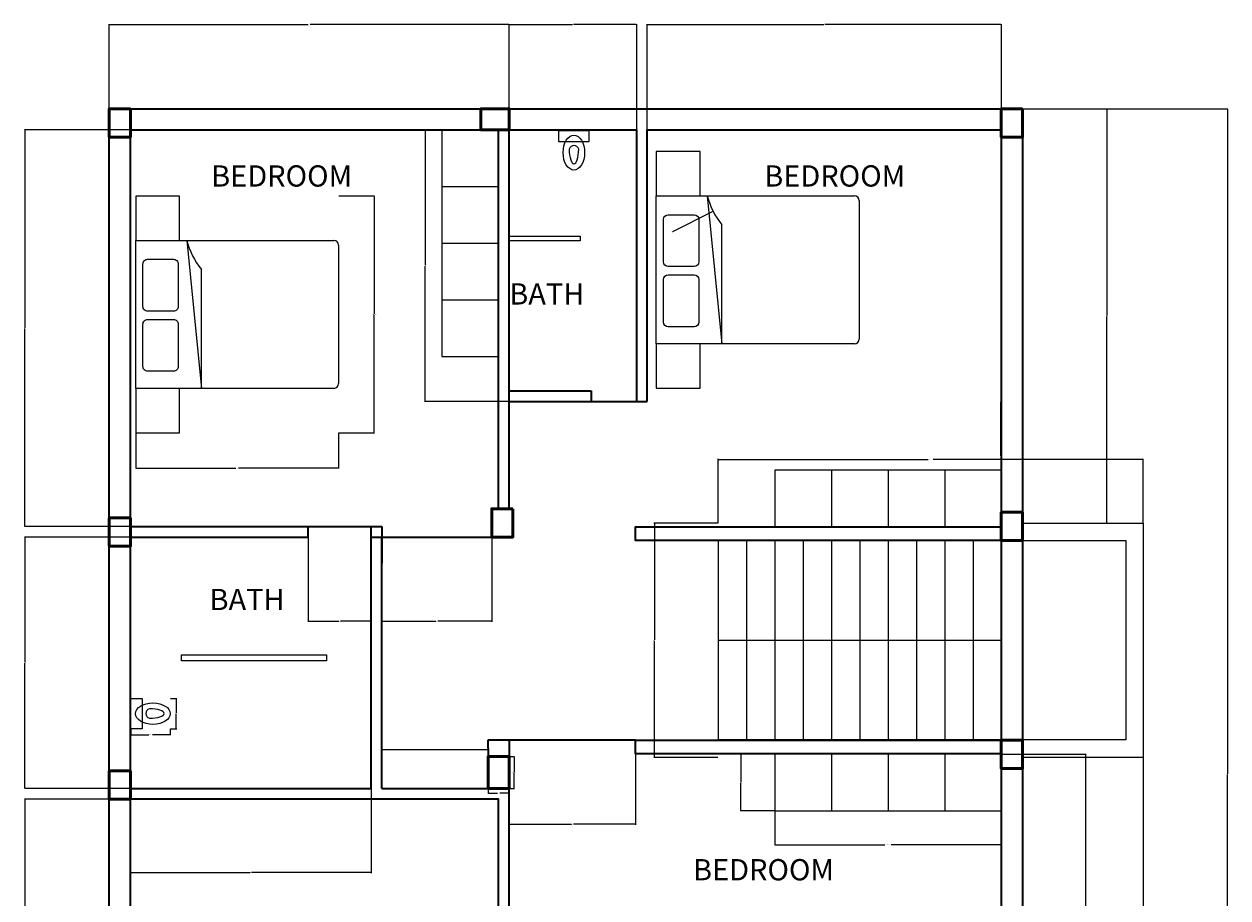
# Model space of a CAD drawing. Units: inches. Extents: x 1748 to 3019, y 1454 to 2188.
# Tile 4 of 4: x 2509 to 3019, y 1818 to 2188. Entities that reach past the tile are written whole.
import ezdxf

# ---------------------------------------------------------------- set-up
doc = ezdxf.new("R2010")
doc.units = ezdxf.units.IN
for name, color, linetype, lineweight in [('A-ANNO-DIMS', 2, 'Continuous', 18), ('A-AREA-IDEN', 134, 'Continuous', 18), ('A-COLS', 120, 'Continuous', 50), ('A-FLOR-CASE', 9, 'Continuous', 18), ('A-WALL', 7, 'Continuous', 35), ('bathroom', 54, 'Continuous', 18), ('bed', 21, 'Continuous', 18), ('cupboard', 201, 'Continuous', 18), ('stairs', 64, 'Continuous', 25)]:
    doc.layers.add(name, color=color, linetype=linetype, lineweight=lineweight)
doc.styles.get("Standard").update_dxf_attribs({"font": 'arial.ttf'})
doc.dimstyles.get("Standard").update_dxf_attribs({"dimtxt": 0.18, "dimasz": 0.18, "dimexe": 0.18, "dimexo": 0.0625, "dimgap": 0.09, "dimtad": 0, "dimtih": 1, "dimtoh": 1, "dimdec": 4, "dimzin": 0, "dimdsep": 46, "dimtxsty": 'Standard', "dimcen": 0.09, "dimadec": 0, "dimazin": 0, "dimtfac": 1, "dimtdec": 4, "dimtofl": 0, "dimtmove": 0, "dimatfit": 3, "dimfxl": 1, "dimtolj": 1, "dimtzin": 0, "dimarcsym": 0})

# ---------------------------------------------------------------- blocks, each defined once
blk = doc.blocks.new('BED-DOUBLE-NIGHTSTANDS')
for p, q in [((0, 81.51), (83.98, 81.51)), ((0, 18.79), (0, 81.51)), ((21.61, 81.51), (27.83, 18.79)), ((85.98, 79.51), (85.98, 20.79)), ((27.83, 18.79), (27.83, 69.19)), ((83.98, 18.79), (0, 18.79))]:
    blk.add_line(p, q)
for points in [[(0, 81.51), (18.52, 81.51), (18.52, 100.3), (0, 100.3)], [(0, 0), (18.52, 0), (18.52, 18.79), (0, 18.79)]]:
    blk.add_lwpolyline(points, close=True)
for points in [[(5.06, 73.49), (16.01, 73.49, -0.414214), (18.01, 71.49), (18.01, 53.51, -0.414214), (16.01, 51.51), (5.06, 51.51, -0.414214), (3.06, 53.51), (3.06, 71.49, -0.414214)], [(5.06, 47.99), (16.01, 47.99, -0.414214), (18.01, 45.99), (18.01, 28.02, -0.414214), (16.01, 26.02), (5.06, 26.02, -0.414214), (3.06, 28.02), (3.06, 45.99, -0.414214)]]:
    blk.add_lwpolyline(points, format="xyb", close=True)
for centre, radius, start, end in [((52.42, 89.31), 31.78, 194.1991, 219.2902), ((83.98, 79.51), 2, 0, 90), ((83.98, 79.51), 2, 0, 90), ((83.98, 20.79), 2, 270, 0)]:
    blk.add_arc(centre, radius, start, end)
blk = doc.blocks.new('WARDROBE-4-BAY')
for p, q in [((24, 96), (0, 96)), ((0, 96), (0, 0)), ((24, 0), (24, 96)), ((0, 72), (24, 72)), ((0, 48), (24, 48)), ((0, 24), (24, 24)), ((0, 0), (24, 0))]:
    blk.add_line(p, q)
blk = doc.blocks.new('WC-CLOSE-COUPLED')
blk.add_lwpolyline([(0, 12.82), (4.89, 12.82), (4.89, 0), (0, 0)], close=True)
blk.add_arc((8.58, 6.47), 2.15, 108.3808, 251.6192)
blk.add_ellipse((9.39, 6.41), major_axis=(7.38, 0), ratio=0.615385)
blk.add_ellipse((7.39, 6.47), major_axis=(6.81, 0), ratio=0.3, start_param=4.786849, end_param=7.779521)
blk = doc.blocks.new('STAIR-FLIGHT-LANDING')
for p, q in [((0, 91.88), (129, 91.88)), ((0, 91.88), (0, 7.38)), ((12, 91.88), (12, 7.38)), ((24, 91.88), (24, 7.38)), ((36, 91.88), (36, 7.38)), ((48, 91.88), (48, 7.38)), ((60, 91.88), (60, 7.38)), ((72, 91.88), (72, 7.38)), ((84, 91.88), (84, 7.38)), ((96, 91.88), (96, 7.38)), ((108, 91.88), (108, 7.38)), ((120, 91.88), (120, 7.38)), ((0, 49.63), (120, 49.63)), ((129, 7.38), (0, 7.38))]:
    blk.add_line(p, q)
blk.add_lwpolyline([(129, 99.26), (180.11, 99.26), (180.11, 0), (129, 0)])
blk.add_lwpolyline([(129, 91.88), (172.73, 91.88), (172.73, 7.38), (129, 7.38)], close=True)
blk = doc.blocks.new('COLUMN-9X12')
blk.add_lwpolyline([(9, 12), (9, 0), (0, 0), (0, 12)], close=True)
blk = doc.blocks.new('COLUMN-RECT-EXTENDED')
blk.add_lwpolyline([(9, 13.44), (9, 0), (0, 0), (0, 13.44)], close=True)
blk = doc.blocks.new('*D10')
at = {"layer": 'A-ANNO-DIMS', "color": 0, "lineweight": -2, "transparency": 16777216}
for p, q in [((2714.2, 1877.38), (2716.33, 1877.38)), ((2716.15, 1877.2), (2716.15, 1870.85)), ((2716.15, 1864.12), (2716.15, 1870.48)), ((2714.2, 1863.94), (2716.33, 1863.94))]:
    blk.add_line(p, q, dxfattribs=at)
at = {"layer": 'A-ANNO-DIMS', "color": 0, "transparency": 16777216}
for points in [[(2716.12, 1877.2), (2716.18, 1877.2), (2716.15, 1877.38)], [(2716.12, 1864.12), (2716.18, 1864.12), (2716.15, 1863.94)]]:
    blk.add_solid(points, dxfattribs=at)
at = {"layer": 'Defpoints', "color": 0, "transparency": 16777216}
for p in [(2714.14, 1877.38), (2716.15, 1877.38), (2714.14, 1863.94)]:
    blk.add_point(p, dxfattribs=at)
at = {"layer": 'A-ANNO-DIMS', "color": 0, "transparency": 16777216, "insert": (2716.15, 1870.66), "char_height": 0.18, "attachment_point": 5}
blk.add_mtext('\\A1;COLUMN 13 TYP.', dxfattribs=at)
blk = doc.blocks.new('*D11')
at = {"layer": 'A-ANNO-DIMS', "color": 0, "lineweight": -2, "transparency": 16777216}
for p, q in [((2705.14, 1863.88), (2705.14, 1861.74)), ((2705.32, 1861.92), (2709.18, 1861.92)), ((2713.96, 1861.92), (2710.09, 1861.92)), ((2714.14, 1863.88), (2714.14, 1861.74))]:
    blk.add_line(p, q, dxfattribs=at)
at = {"layer": 'A-ANNO-DIMS', "color": 0, "transparency": 16777216}
for points in [[(2705.32, 1861.95), (2705.32, 1861.89), (2705.14, 1861.92)], [(2713.96, 1861.95), (2713.96, 1861.89), (2714.14, 1861.92)]]:
    blk.add_solid(points, dxfattribs=at)
at = {"layer": 'Defpoints', "color": 0, "transparency": 16777216}
for p in [(2705.14, 1863.94), (2714.14, 1863.94), (2714.14, 1861.92)]:
    blk.add_point(p, dxfattribs=at)
at = {"layer": 'A-ANNO-DIMS', "color": 0, "transparency": 16777216, "insert": (2709.64, 1861.92), "char_height": 0.18, "attachment_point": 5}
blk.add_mtext('\\A1;9 TYP.', dxfattribs=at)
blk = doc.blocks.new('*D12')
at = {"layer": 'A-ANNO-DIMS', "color": 0, "lineweight": -2, "transparency": 16777216}
for p, q in [((2826.64, 1854.35), (2826.64, 1839.83)), ((2922.64, 1854.35), (2922.64, 1839.83)), ((2826.82, 1840.01), (2873.33, 1840.01)), ((2922.46, 1840.01), (2875.94, 1840.01))]:
    blk.add_line(p, q, dxfattribs=at)
at = {"layer": 'A-ANNO-DIMS', "color": 0, "transparency": 16777216}
for points in [[(2826.82, 1840.04), (2826.82, 1839.98), (2826.64, 1840.01)], [(2922.46, 1840.04), (2922.46, 1839.98), (2922.64, 1840.01)]]:
    blk.add_solid(points, dxfattribs=at)
at = {"layer": 'Defpoints', "color": 0, "transparency": 16777216}
for p in [(2826.64, 1854.41), (2922.64, 1854.41), (2922.64, 1840.01)]:
    blk.add_point(p, dxfattribs=at)
at = {"layer": 'A-ANNO-DIMS', "color": 0, "transparency": 16777216, "insert": (2874.64, 1840.01), "char_height": 0.18, "attachment_point": 5}
blk.add_mtext('\\A1;WARDROBE 96 TYP.', dxfattribs=at)
blk = doc.blocks.new('*D13')
at = {"layer": 'A-ANNO-DIMS', "color": 0, "lineweight": -2, "transparency": 16777216}
for p, q in [((2826.57, 1878.41), (2812.06, 1878.41)), ((2812.24, 1878.23), (2812.24, 1866.59)), ((2812.24, 1854.59), (2812.24, 1866.23)), ((2826.57, 1854.41), (2812.06, 1854.41))]:
    blk.add_line(p, q, dxfattribs=at)
at = {"layer": 'A-ANNO-DIMS', "color": 0, "transparency": 16777216}
for points in [[(2812.21, 1878.23), (2812.27, 1878.23), (2812.24, 1878.41)], [(2812.21, 1854.59), (2812.27, 1854.59), (2812.24, 1854.41)]]:
    blk.add_solid(points, dxfattribs=at)
at = {"layer": 'Defpoints', "color": 0, "transparency": 16777216}
for p in [(2826.64, 1878.41), (2812.24, 1854.41), (2826.64, 1854.41)]:
    blk.add_point(p, dxfattribs=at)
at = {"layer": 'A-ANNO-DIMS', "color": 0, "transparency": 16777216, "insert": (2812.24, 1866.41), "char_height": 0.18, "attachment_point": 5}
blk.add_mtext('\\A1;24 TYP.', dxfattribs=at)
blk = doc.blocks.new('*D14')
at = {"layer": 'A-ANNO-DIMS', "color": 0, "lineweight": -2, "transparency": 16777216}
for p, q in [((2553.76, 1889.14), (2553.76, 1886.51)), ((2570.53, 1889.14), (2570.53, 1886.51)), ((2553.94, 1886.69), (2561.37, 1886.69)), ((2570.35, 1886.69), (2562.92, 1886.69))]:
    blk.add_line(p, q, dxfattribs=at)
at = {"layer": 'A-ANNO-DIMS', "color": 0, "transparency": 16777216}
for points in [[(2553.94, 1886.72), (2553.94, 1886.66), (2553.76, 1886.69)], [(2570.35, 1886.72), (2570.35, 1886.66), (2570.53, 1886.69)]]:
    blk.add_solid(points, dxfattribs=at)
at = {"layer": 'Defpoints', "color": 0, "transparency": 16777216}
for p in [(2553.76, 1889.2), (2570.53, 1889.2), (2570.53, 1886.69)]:
    blk.add_point(p, dxfattribs=at)
at = {"layer": 'A-ANNO-DIMS', "color": 0, "transparency": 16777216, "insert": (2562.14, 1886.69), "char_height": 0.18, "attachment_point": 5}
blk.add_mtext('\\A1;WC 17 TYP.', dxfattribs=at)
blk = doc.blocks.new('*D15')
at = {"layer": 'A-ANNO-DIMS', "color": 0, "lineweight": -2, "transparency": 16777216}
for p, q in [((2570.59, 1902.02), (2573.22, 1902.02)), ((2573.04, 1901.84), (2573.04, 1895.8)), ((2573.04, 1889.38), (2573.04, 1895.43)), ((2570.59, 1889.2), (2573.22, 1889.2))]:
    blk.add_line(p, q, dxfattribs=at)
at = {"layer": 'A-ANNO-DIMS', "color": 0, "transparency": 16777216}
for points in [[(2573.01, 1901.84), (2573.07, 1901.84), (2573.04, 1902.02)], [(2573.01, 1889.38), (2573.07, 1889.38), (2573.04, 1889.2)]]:
    blk.add_solid(points, dxfattribs=at)
at = {"layer": 'Defpoints', "color": 0, "transparency": 16777216}
for p in [(2570.53, 1902.02), (2573.04, 1902.02), (2570.53, 1889.2)]:
    blk.add_point(p, dxfattribs=at)
at = {"layer": 'A-ANNO-DIMS', "color": 0, "transparency": 16777216, "insert": (2573.04, 1895.61), "char_height": 0.18, "attachment_point": 5}
blk.add_mtext('\\A1;13 TYP.', dxfattribs=at)
blk = doc.blocks.new('*D18')
at = {"layer": 'A-ANNO-DIMS', "color": 0, "lineweight": -2, "transparency": 16777216}
for p, q in [((2641.9, 2114.97), (2657.07, 2114.97)), ((2656.89, 2114.79), (2656.89, 2065)), ((2656.89, 2014.84), (2656.89, 2064.63)), ((2641.9, 2014.66), (2657.07, 2014.66))]:
    blk.add_line(p, q, dxfattribs=at)
at = {"layer": 'A-ANNO-DIMS', "color": 0, "transparency": 16777216}
for points in [[(2656.86, 2114.79), (2656.92, 2114.79), (2656.89, 2114.97)], [(2656.86, 2014.84), (2656.92, 2014.84), (2656.89, 2014.66)]]:
    blk.add_solid(points, dxfattribs=at)
at = {"layer": 'Defpoints', "color": 0, "transparency": 16777216}
for p in [(2641.84, 2114.97), (2656.89, 2114.97), (2641.84, 2014.66)]:
    blk.add_point(p, dxfattribs=at)
at = {"layer": 'A-ANNO-DIMS', "color": 0, "transparency": 16777216, "insert": (2656.89, 2064.81), "char_height": 0.18, "attachment_point": 5}
blk.add_mtext('\\A1;BED SET 100 TYP.', dxfattribs=at)
blk = doc.blocks.new('*D19')
at = {"layer": 'A-ANNO-DIMS', "color": 0, "lineweight": -2, "transparency": 16777216}
for p, q in [((2555.86, 2014.6), (2555.86, 1999.44)), ((2641.84, 2014.6), (2641.84, 1999.44)), ((2556.04, 1999.62), (2598.32, 1999.62)), ((2641.66, 1999.62), (2599.38, 1999.62))]:
    blk.add_line(p, q, dxfattribs=at)
at = {"layer": 'A-ANNO-DIMS', "color": 0, "transparency": 16777216}
for points in [[(2556.04, 1999.65), (2556.04, 1999.59), (2555.86, 1999.62)], [(2641.66, 1999.65), (2641.66, 1999.59), (2641.84, 1999.62)]]:
    blk.add_solid(points, dxfattribs=at)
at = {"layer": 'Defpoints', "color": 0, "transparency": 16777216}
for p in [(2555.86, 2014.66), (2641.84, 2014.66), (2641.84, 1999.62)]:
    blk.add_point(p, dxfattribs=at)
at = {"layer": 'A-ANNO-DIMS', "color": 0, "transparency": 16777216, "insert": (2598.85, 1999.62), "char_height": 0.18, "attachment_point": 5}
blk.add_mtext('\\A1;86 TYP.', dxfattribs=at)
blk = doc.blocks.new('*D20')
at = {"layer": 'A-ANNO-DIMS', "color": 0, "lineweight": -2, "transparency": 16777216}
for p, q in [((2802.64, 1976.38), (2802.64, 2003.52)), ((2802.82, 2003.34), (2891.69, 2003.34)), ((2982.56, 2003.34), (2893.69, 2003.34)), ((2982.74, 1976.38), (2982.74, 2003.52))]:
    blk.add_line(p, q, dxfattribs=at)
at = {"layer": 'A-ANNO-DIMS', "color": 0, "transparency": 16777216}
for points in [[(2802.82, 2003.37), (2802.82, 2003.31), (2802.64, 2003.34)], [(2982.56, 2003.37), (2982.56, 2003.31), (2982.74, 2003.34)]]:
    blk.add_solid(points, dxfattribs=at)
at = {"layer": 'Defpoints', "color": 0, "transparency": 16777216}
for p in [(2982.74, 2003.34), (2802.64, 1976.32), (2982.74, 1976.32)]:
    blk.add_point(p, dxfattribs=at)
at = {"layer": 'A-ANNO-DIMS', "color": 0, "transparency": 16777216, "insert": (2892.69, 2003.34), "char_height": 0.18, "attachment_point": 5}
blk.add_mtext('\\A1;STAIR 180 TYP.', dxfattribs=at)
blk = doc.blocks.new('*D21')
at = {"layer": 'A-ANNO-DIMS', "color": 0, "lineweight": -2, "transparency": 16777216}
for p, q in [((2802.57, 1976.32), (2775.44, 1976.32)), ((2775.62, 1976.14), (2775.62, 1926.87)), ((2775.62, 1877.24), (2775.62, 1926.51)), ((2802.57, 1877.06), (2775.44, 1877.06))]:
    blk.add_line(p, q, dxfattribs=at)
at = {"layer": 'A-ANNO-DIMS', "color": 0, "transparency": 16777216}
for points in [[(2775.59, 1976.14), (2775.65, 1976.14), (2775.62, 1976.32)], [(2775.59, 1877.24), (2775.65, 1877.24), (2775.62, 1877.06)]]:
    blk.add_solid(points, dxfattribs=at)
at = {"layer": 'Defpoints', "color": 0, "transparency": 16777216}
for p in [(2775.62, 1976.32), (2802.64, 1976.32), (2802.64, 1877.06)]:
    blk.add_point(p, dxfattribs=at)
at = {"layer": 'A-ANNO-DIMS', "color": 0, "transparency": 16777216, "insert": (2775.62, 1926.69), "char_height": 0.18, "attachment_point": 5}
blk.add_mtext('\\A1;99 TYP.', dxfattribs=at)
blk = doc.blocks.new('*D44')
at = {"layer": 'A-ANNO-DIMS', "color": 0, "lineweight": -2, "transparency": 16777216}
for p, q in [((2982.74, 1877), (2982.74, 1552.06)), ((2544.64, 1587.88), (2544.64, 1552.06)), ((2544.82, 1552.24), (2763.31, 1552.24)), ((2982.56, 1552.24), (2764.07, 1552.24))]:
    blk.add_line(p, q, dxfattribs=at)
at = {"layer": 'A-ANNO-DIMS', "color": 0, "transparency": 16777216}
for points in [[(2544.82, 1552.27), (2544.82, 1552.21), (2544.64, 1552.24)], [(2982.56, 1552.27), (2982.56, 1552.21), (2982.74, 1552.24)]]:
    blk.add_solid(points, dxfattribs=at)
at = {"layer": 'Defpoints', "color": 0, "transparency": 16777216}
for p in [(2982.74, 1877.06), (2544.64, 1587.94), (2982.74, 1552.24)]:
    blk.add_point(p, dxfattribs=at)
at = {"layer": 'A-ANNO-DIMS', "color": 0, "transparency": 16777216, "insert": (2763.69, 1552.24), "char_height": 0.18, "attachment_point": 5}
blk.add_mtext('\\A1;438.1', dxfattribs=at)
blk = doc.blocks.new('*D45')
at = {"layer": 'A-ANNO-DIMS', "color": 0, "lineweight": -2, "transparency": 16777216}
for p, q in [((2931.7, 2151.94), (3018.62, 2151.94)), ((3018.44, 2151.76), (3018.44, 1870.12)), ((3018.44, 1588.12), (3018.44, 1869.76)), ((2886.7, 1587.94), (3018.62, 1587.94))]:
    blk.add_line(p, q, dxfattribs=at)
at = {"layer": 'A-ANNO-DIMS', "color": 0, "transparency": 16777216}
for points in [[(3018.41, 2151.76), (3018.47, 2151.76), (3018.44, 2151.94)], [(3018.41, 1588.12), (3018.47, 1588.12), (3018.44, 1587.94)]]:
    blk.add_solid(points, dxfattribs=at)
at = {"layer": 'Defpoints', "color": 0, "transparency": 16777216}
for p in [(2931.64, 2151.94), (3018.44, 2151.94), (2886.64, 1587.94)]:
    blk.add_point(p, dxfattribs=at)
at = {"layer": 'A-ANNO-DIMS', "color": 0, "transparency": 16777216, "insert": (3018.44, 1869.94), "char_height": 0.18, "attachment_point": 5}
blk.add_mtext('\\A1;564', dxfattribs=at)
blk = doc.blocks.new('*D46')
at = {"layer": 'A-ANNO-DIMS', "color": 0, "lineweight": -2, "transparency": 16777216}
for p, q in [((2544.64, 2152), (2544.64, 2187.82)), ((2544.82, 2187.64), (2629, 2187.64)), ((2713.96, 2187.64), (2629.77, 2187.64)), ((2714.14, 2152), (2714.14, 2187.82))]:
    blk.add_line(p, q, dxfattribs=at)
at = {"layer": 'A-ANNO-DIMS', "color": 0, "transparency": 16777216}
for points in [[(2544.82, 2187.67), (2544.82, 2187.61), (2544.64, 2187.64)], [(2713.96, 2187.67), (2713.96, 2187.61), (2714.14, 2187.64)]]:
    blk.add_solid(points, dxfattribs=at)
at = {"layer": 'Defpoints', "color": 0, "transparency": 16777216}
for p in [(2714.14, 2187.64), (2544.64, 2151.94), (2714.14, 2151.94)]:
    blk.add_point(p, dxfattribs=at)
at = {"layer": 'A-ANNO-DIMS', "color": 0, "transparency": 16777216, "insert": (2629.39, 2187.64), "char_height": 0.18, "attachment_point": 5}
blk.add_mtext('\\A1;169.5', dxfattribs=at)
blk = doc.blocks.new('*D47')
at = {"layer": 'A-ANNO-DIMS', "color": 0, "lineweight": -2, "transparency": 16777216}
for p, q in [((2714.14, 2143), (2714.14, 2187.82)), ((2714.32, 2187.64), (2740.92, 2187.64)), ((2767.96, 2187.64), (2741.35, 2187.64)), ((2768.14, 2143), (2768.14, 2187.82))]:
    blk.add_line(p, q, dxfattribs=at)
at = {"layer": 'A-ANNO-DIMS', "color": 0, "transparency": 16777216}
for points in [[(2714.32, 2187.67), (2714.32, 2187.61), (2714.14, 2187.64)], [(2767.96, 2187.67), (2767.96, 2187.61), (2768.14, 2187.64)]]:
    blk.add_solid(points, dxfattribs=at)
at = {"layer": 'Defpoints', "color": 0, "transparency": 16777216}
for p in [(2768.14, 2187.64), (2714.14, 2142.94), (2768.14, 2142.94)]:
    blk.add_point(p, dxfattribs=at)
at = {"layer": 'A-ANNO-DIMS', "color": 0, "transparency": 16777216, "insert": (2741.14, 2187.64), "char_height": 0.18, "attachment_point": 5}
blk.add_mtext('\\A1;54', dxfattribs=at)
blk = doc.blocks.new('*D48')
at = {"layer": 'A-ANNO-DIMS', "color": 0, "lineweight": -2, "transparency": 16777216}
for p, q in [((2772.64, 2143.03), (2772.64, 2187.82)), ((2772.82, 2187.64), (2847.36, 2187.64)), ((2922.46, 2187.64), (2847.92, 2187.64)), ((2922.64, 2143), (2922.64, 2187.82))]:
    blk.add_line(p, q, dxfattribs=at)
at = {"layer": 'A-ANNO-DIMS', "color": 0, "transparency": 16777216}
for points in [[(2772.82, 2187.67), (2772.82, 2187.61), (2772.64, 2187.64)], [(2922.46, 2187.67), (2922.46, 2187.61), (2922.64, 2187.64)]]:
    blk.add_solid(points, dxfattribs=at)
at = {"layer": 'Defpoints', "color": 0, "transparency": 16777216}
for p in [(2922.64, 2187.64), (2772.64, 2142.97), (2922.64, 2142.94)]:
    blk.add_point(p, dxfattribs=at)
at = {"layer": 'A-ANNO-DIMS', "color": 0, "transparency": 16777216, "insert": (2847.64, 2187.64), "char_height": 0.18, "attachment_point": 5}
blk.add_mtext('\\A1;150', dxfattribs=at)
blk = doc.blocks.new('*D49')
at = {"layer": 'A-ANNO-DIMS', "color": 0, "lineweight": -2, "transparency": 16777216}
for p, q in [((2714.07, 2142.94), (2678.26, 2142.94)), ((2678.44, 2142.76), (2678.44, 2085.59)), ((2678.44, 2028.05), (2678.44, 2085.22)), ((2714.07, 2027.87), (2678.26, 2027.87))]:
    blk.add_line(p, q, dxfattribs=at)
at = {"layer": 'A-ANNO-DIMS', "color": 0, "transparency": 16777216}
for points in [[(2678.41, 2142.76), (2678.47, 2142.76), (2678.44, 2142.94)], [(2678.41, 2028.05), (2678.47, 2028.05), (2678.44, 2027.87)]]:
    blk.add_solid(points, dxfattribs=at)
at = {"layer": 'Defpoints', "color": 0, "transparency": 16777216}
for p in [(2678.44, 2142.94), (2714.14, 2142.94), (2714.14, 2027.87)]:
    blk.add_point(p, dxfattribs=at)
at = {"layer": 'A-ANNO-DIMS', "color": 0, "transparency": 16777216, "insert": (2678.44, 2085.4), "char_height": 0.18, "attachment_point": 5}
blk.add_mtext('\\A1;115.07', dxfattribs=at)
blk = doc.blocks.new('*D50')
at = {"layer": 'A-ANNO-DIMS', "color": 0, "lineweight": -2, "transparency": 16777216}
for p, q in [((2553.57, 2142.94), (2508.76, 2142.94)), ((2508.94, 2142.76), (2508.94, 2059.12)), ((2508.94, 1975.12), (2508.94, 2058.76)), ((2553.57, 1974.94), (2508.76, 1974.94))]:
    blk.add_line(p, q, dxfattribs=at)
at = {"layer": 'A-ANNO-DIMS', "color": 0, "transparency": 16777216}
for points in [[(2508.91, 2142.76), (2508.97, 2142.76), (2508.94, 2142.94)], [(2508.91, 1975.12), (2508.97, 1975.12), (2508.94, 1974.94)]]:
    blk.add_solid(points, dxfattribs=at)
at = {"layer": 'Defpoints', "color": 0, "transparency": 16777216}
for p in [(2508.94, 2142.94), (2553.64, 2142.94), (2553.64, 1974.94)]:
    blk.add_point(p, dxfattribs=at)
at = {"layer": 'A-ANNO-DIMS', "color": 0, "transparency": 16777216, "insert": (2508.94, 2058.94), "char_height": 0.18, "attachment_point": 5}
blk.add_mtext('\\A1;168', dxfattribs=at)
blk = doc.blocks.new('*D51')
at = {"layer": 'A-ANNO-DIMS', "color": 0, "lineweight": -2, "transparency": 16777216}
for p, q in [((2553.64, 1863.88), (2553.64, 1828.06)), ((2655.64, 1863.88), (2655.64, 1828.06)), ((2553.82, 1828.24), (2604.36, 1828.24)), ((2655.46, 1828.24), (2604.91, 1828.24))]:
    blk.add_line(p, q, dxfattribs=at)
at = {"layer": 'A-ANNO-DIMS', "color": 0, "transparency": 16777216}
for points in [[(2553.82, 1828.27), (2553.82, 1828.21), (2553.64, 1828.24)], [(2655.46, 1828.27), (2655.46, 1828.21), (2655.64, 1828.24)]]:
    blk.add_solid(points, dxfattribs=at)
at = {"layer": 'Defpoints', "color": 0, "transparency": 16777216}
for p in [(2553.64, 1863.94), (2655.64, 1863.94), (2553.64, 1828.24)]:
    blk.add_point(p, dxfattribs=at)
at = {"layer": 'A-ANNO-DIMS', "color": 0, "transparency": 16777216, "insert": (2604.64, 1828.24), "char_height": 0.18, "attachment_point": 5}
blk.add_mtext('\\A1;102', dxfattribs=at)
blk = doc.blocks.new('*D52')
at = {"layer": 'A-ANNO-DIMS', "color": 0, "lineweight": -2, "transparency": 16777216}
for p, q in [((2553.57, 1970.44), (2508.76, 1970.44)), ((2508.94, 1970.26), (2508.94, 1917.37)), ((2508.94, 1864.12), (2508.94, 1917.01)), ((2553.57, 1863.94), (2508.76, 1863.94))]:
    blk.add_line(p, q, dxfattribs=at)
at = {"layer": 'A-ANNO-DIMS', "color": 0, "transparency": 16777216}
for points in [[(2508.91, 1970.26), (2508.97, 1970.26), (2508.94, 1970.44)], [(2508.91, 1864.12), (2508.97, 1864.12), (2508.94, 1863.94)]]:
    blk.add_solid(points, dxfattribs=at)
at = {"layer": 'Defpoints', "color": 0, "transparency": 16777216}
for p in [(2508.94, 1970.44), (2553.64, 1970.44), (2553.64, 1863.94)]:
    blk.add_point(p, dxfattribs=at)
at = {"layer": 'A-ANNO-DIMS', "color": 0, "transparency": 16777216, "insert": (2508.94, 1917.19), "char_height": 0.18, "attachment_point": 5}
blk.add_mtext('\\A1;106.5', dxfattribs=at)
blk = doc.blocks.new('*D53')
at = {"layer": 'A-ANNO-DIMS', "color": 0, "lineweight": -2, "transparency": 16777216}
for p, q in [((2544.57, 1859.39), (2508.76, 1859.39)), ((2508.94, 1859.21), (2508.94, 1763.6)), ((2508.94, 1667.62), (2508.94, 1763.23)), ((2544.57, 1667.44), (2508.76, 1667.44))]:
    blk.add_line(p, q, dxfattribs=at)
at = {"layer": 'A-ANNO-DIMS', "color": 0, "transparency": 16777216}
for points in [[(2508.91, 1859.21), (2508.97, 1859.21), (2508.94, 1859.39)], [(2508.91, 1667.62), (2508.97, 1667.62), (2508.94, 1667.44)]]:
    blk.add_solid(points, dxfattribs=at)
at = {"layer": 'Defpoints', "color": 0, "transparency": 16777216}
for p in [(2508.94, 1859.39), (2544.64, 1859.39), (2544.64, 1667.44)]:
    blk.add_point(p, dxfattribs=at)
at = {"layer": 'A-ANNO-DIMS', "color": 0, "transparency": 16777216, "insert": (2508.94, 1763.42), "char_height": 0.18, "attachment_point": 5}
blk.add_mtext('\\A1;191.95', dxfattribs=at)
blk = doc.blocks.new('*D55')
at = {"layer": 'A-ANNO-DIMS', "color": 0, "lineweight": -2, "transparency": 16777216}
for p, q in [((2922.7, 1878.41), (2958.52, 1878.41)), ((2958.34, 1878.23), (2958.34, 1794.11)), ((2958.34, 1709.62), (2958.34, 1793.74)), ((2922.7, 1709.44), (2958.52, 1709.44))]:
    blk.add_line(p, q, dxfattribs=at)
at = {"layer": 'A-ANNO-DIMS', "color": 0, "transparency": 16777216}
for points in [[(2958.31, 1878.23), (2958.37, 1878.23), (2958.34, 1878.41)], [(2958.31, 1709.62), (2958.37, 1709.62), (2958.34, 1709.44)]]:
    blk.add_solid(points, dxfattribs=at)
at = {"layer": 'Defpoints', "color": 0, "transparency": 16777216}
for p in [(2922.64, 1878.41), (2922.64, 1709.44), (2958.34, 1709.44)]:
    blk.add_point(p, dxfattribs=at)
at = {"layer": 'A-ANNO-DIMS', "color": 0, "transparency": 16777216, "insert": (2958.34, 1793.93), "char_height": 0.18, "attachment_point": 5}
blk.add_mtext('\\A1;168.97', dxfattribs=at)
blk = doc.blocks.new('*D61')
at = {"layer": 'A-ANNO-DIMS', "color": 0, "lineweight": -2, "transparency": 16777216}
for p, q in [((2931.7, 2151.94), (2967.52, 2151.94)), ((2967.34, 2151.76), (2967.34, 2064.31)), ((2967.34, 1976.5), (2967.34, 2063.95)), ((2931.7, 1976.32), (2967.52, 1976.32))]:
    blk.add_line(p, q, dxfattribs=at)
at = {"layer": 'A-ANNO-DIMS', "color": 0, "transparency": 16777216}
for points in [[(2967.31, 2151.76), (2967.37, 2151.76), (2967.34, 2151.94)], [(2967.31, 1976.5), (2967.37, 1976.5), (2967.34, 1976.32)]]:
    blk.add_solid(points, dxfattribs=at)
at = {"layer": 'Defpoints', "color": 0, "transparency": 16777216}
for p in [(2931.64, 2151.94), (2931.64, 1976.32), (2967.34, 1976.32)]:
    blk.add_point(p, dxfattribs=at)
at = {"layer": 'A-ANNO-DIMS', "color": 0, "transparency": 16777216, "insert": (2967.34, 2064.13), "char_height": 0.18, "attachment_point": 5}
blk.add_mtext('\\A1;175.62', dxfattribs=at)
blk = doc.blocks.new('*D62')
at = {"layer": 'A-ANNO-DIMS', "color": 0, "lineweight": -2, "transparency": 16777216}
for p, q in [((2628.91, 1970.38), (2628.91, 1934.56)), ((2655.64, 1970.38), (2655.64, 1934.56)), ((2629.09, 1934.74), (2641.88, 1934.74)), ((2655.46, 1934.74), (2642.67, 1934.74))]:
    blk.add_line(p, q, dxfattribs=at)
at = {"layer": 'A-ANNO-DIMS', "color": 0, "transparency": 16777216}
for points in [[(2629.09, 1934.77), (2629.09, 1934.71), (2628.91, 1934.74)], [(2655.46, 1934.77), (2655.46, 1934.71), (2655.64, 1934.74)]]:
    blk.add_solid(points, dxfattribs=at)
at = {"layer": 'Defpoints', "color": 0, "transparency": 16777216}
for p in [(2628.91, 1970.44), (2655.64, 1970.44), (2628.91, 1934.74)]:
    blk.add_point(p, dxfattribs=at)
at = {"layer": 'A-ANNO-DIMS', "color": 0, "transparency": 16777216, "insert": (2642.27, 1934.74), "char_height": 0.18, "attachment_point": 5}
blk.add_mtext('\\A1;26.72', dxfattribs=at)
blk = doc.blocks.new('*D63')
at = {"layer": 'A-ANNO-DIMS', "color": 0, "lineweight": -2, "transparency": 16777216}
for p, q in [((2660.14, 1970.38), (2660.14, 1934.56)), ((2706.69, 1970.38), (2706.69, 1934.56)), ((2660.32, 1934.74), (2683.01, 1934.74)), ((2706.51, 1934.74), (2683.81, 1934.74))]:
    blk.add_line(p, q, dxfattribs=at)
at = {"layer": 'A-ANNO-DIMS', "color": 0, "transparency": 16777216}
for points in [[(2660.32, 1934.77), (2660.32, 1934.71), (2660.14, 1934.74)], [(2706.51, 1934.77), (2706.51, 1934.71), (2706.69, 1934.74)]]:
    blk.add_solid(points, dxfattribs=at)
at = {"layer": 'Defpoints', "color": 0, "transparency": 16777216}
for p in [(2660.14, 1970.44), (2706.69, 1970.44), (2660.14, 1934.74)]:
    blk.add_point(p, dxfattribs=at)
at = {"layer": 'A-ANNO-DIMS', "color": 0, "transparency": 16777216, "insert": (2683.41, 1934.74), "char_height": 0.18, "attachment_point": 5}
blk.add_mtext('\\A1;46.55', dxfattribs=at)
blk = doc.blocks.new('*D64')
at = {"layer": 'A-ANNO-DIMS', "color": 0, "lineweight": -2, "transparency": 16777216}
for p, q in [((2714.14, 1884.35), (2714.14, 1848.53)), ((2767.68, 1884.35), (2767.68, 1848.53)), ((2714.32, 1848.71), (2740.51, 1848.71)), ((2767.5, 1848.71), (2741.3, 1848.71))]:
    blk.add_line(p, q, dxfattribs=at)
at = {"layer": 'A-ANNO-DIMS', "color": 0, "transparency": 16777216}
for points in [[(2714.32, 1848.74), (2714.32, 1848.68), (2714.14, 1848.71)], [(2767.5, 1848.74), (2767.5, 1848.68), (2767.68, 1848.71)]]:
    blk.add_solid(points, dxfattribs=at)
at = {"layer": 'Defpoints', "color": 0, "transparency": 16777216}
for p in [(2714.14, 1884.41), (2767.68, 1884.41), (2714.14, 1848.71)]:
    blk.add_point(p, dxfattribs=at)
at = {"layer": 'A-ANNO-DIMS', "color": 0, "transparency": 16777216, "insert": (2740.91, 1848.71), "char_height": 0.18, "attachment_point": 5}
blk.add_mtext('\\A1;53.54', dxfattribs=at)
blk = doc.blocks.new('*D69')
at = {"layer": 'A-ANNO-DIMS', "color": 0, "lineweight": -2, "transparency": 16777216}
for p, q in [((2828.77, 2122.84), (2828.95, 2122.84)), ((2828.86, 2122.75), (2828.86, 2122.93)), ((2783.45, 2099.96), (2800.32, 2108.46)), ((2783.27, 2099.96), (2783.45, 2099.96))]:
    blk.add_line(p, q, dxfattribs=at)
at = {"layer": 'A-ANNO-DIMS', "color": 0, "transparency": 16777216}
blk.add_solid([(2800.31, 2108.49), (2800.33, 2108.43), (2800.48, 2108.54)], dxfattribs=at)
at = {"layer": 'Defpoints', "color": 0, "transparency": 16777216}
for p in [(2828.86, 2122.84), (2800.48, 2108.54)]:
    blk.add_point(p, dxfattribs=at)
at = {"layer": 'A-ANNO-DIMS', "color": 0, "transparency": 16777216, "insert": (2782.6, 2099.96), "char_height": 0.18, "attachment_point": 5}
blk.add_mtext('\\A1;3X R31.78', dxfattribs=at)

msp = doc.modelspace()

# ---------------------------------------------------------------- linework, layer by layer
at = {"layer": 'A-FLOR-CASE'}
msp.add_line((2705.1292, 1880.2386), (2660.1353, 1880.2386), dxfattribs=at)
at = {"layer": 'A-WALL'}
for p, q in [((2553.6353, 2142.94), (2709.6353, 2142.94)), ((2553.6353, 1974.94), (2553.6353, 2142.94)), ((2709.6353, 1982.44), (2709.6353, 2142.94)), ((2714.1353, 2142.94), (2768.1353, 2142.94)), ((2714.1353, 2052.94), (2714.1353, 2142.94)), ((2768.1353, 2027.8673), (2768.1353, 2142.94)), ((2772.6353, 2027.8673), (2772.6353, 2142.9677)), ((2772.6353, 2142.9677), (2922.6353, 2142.9677)), ((2822.1836, 2142.94), (2822.1836, 2142.9677)), ((2922.6353, 2142.94), (2922.6353, 1709.44)), ((2714.1353, 1982.44), (2714.1353, 2052.94)), ((2714.1353, 2032.3673), (2748.8656, 2032.3673)), ((2748.8656, 2032.3673), (2748.8656, 2027.8673)), ((2714.1353, 2027.8673), (2772.6353, 2027.8673)), ((2714.1353, 2026.1397), (2714.1353, 2026.1397)), ((2553.6353, 1974.94), (2660.1353, 1974.94)), ((2628.9144, 1970.44), (2628.9144, 1974.94)), ((2655.6353, 1919.44), (2655.6353, 1974.94)), ((2660.1353, 1974.94), (2660.1353, 1959.3034)), ((2553.6353, 1970.44), (2618.1353, 1970.44)), ((2553.6353, 1919.44), (2553.6353, 1970.44)), ((2618.1353, 1970.44), (2628.9144, 1970.44)), ((2655.6353, 1970.44), (2714.1353, 1970.44)), ((2660.1353, 1919.44), (2660.1353, 1970.44)), ((2553.6353, 1863.94), (2553.6353, 1919.44)), ((2655.6353, 1863.94), (2655.6353, 1919.44)), ((2660.1353, 1863.94), (2660.1353, 1919.44)), ((2767.6791, 1884.412), (2705.1203, 1884.412)), ((2705.1203, 1884.412), (2705.1353, 1877.3845)), ((2714.1353, 1884.412), (2714.1353, 1877.3845)), ((2553.6353, 1863.94), (2655.6353, 1863.94)), ((2660.1353, 1863.94), (2714.1353, 1863.94)), ((2714.1353, 1716.94), (2714.1353, 1863.94)), ((2553.6353, 1859.44), (2709.6353, 1859.44)), ((2553.6353, 1667.44), (2553.6353, 1859.44)), ((2709.6353, 1587.94), (2709.6353, 1859.44))]:
    msp.add_line(p, q, dxfattribs=at)
msp.add_lwpolyline([(2886.6353, 1587.94), (2544.6353, 1587.94), (2544.6353, 2151.94), (2931.6353, 2151.94), (2931.6353, 1709.44)], dxfattribs=at)
for points in [[(2922.6353, 2027.8069), (2922.6353, 2027.8069), (2922.6353, 2004.8656), (2922.6353, 2004.8656)], [(2922.6353, 1968.94), (2767.6791, 1968.94), (2767.6791, 1974.7972), (2922.6353, 1974.7972)], [(2922.6353, 1878.5549), (2767.6791, 1878.5549), (2767.6791, 1884.412), (2922.6353, 1884.412)]]:
    msp.add_lwpolyline(points, close=True, dxfattribs=at)
at = {"layer": 'bathroom'}
for p, q in [((2714.1353, 2097.94), (2744.189, 2097.94)), ((2744.189, 2097.94), (2744.189, 2095.9804)), ((2744.189, 2095.9804), (2714.1353, 2095.9804))]:
    msp.add_line(p, q, dxfattribs=at)
msp.add_lwpolyline([(2575.2445, 1920.5791), (2636.6636, 1920.5791), (2636.6636, 1917.9975), (2575.2445, 1917.9975)], close=True, dxfattribs=at)
at = {"layer": 'bed'}
for p, q in [((2776.4369, 2115.0478), (2860.4191, 2115.0478)), ((2776.4369, 2052.3237), (2776.4369, 2115.0478)), ((2798.0507, 2115.0478), (2804.2632, 2052.3237)), ((2862.4191, 2113.0478), (2862.4191, 2054.3237)), ((2804.2632, 2052.3237), (2804.2632, 2102.7197)), ((2860.4191, 2052.3237), (2776.4369, 2052.3237))]:
    msp.add_line(p, q, dxfattribs=at)
for points in [[(2776.4369, 2115.0478), (2794.9604, 2115.0478), (2794.9604, 2133.8374), (2776.4369, 2133.8374)], [(2776.4369, 2033.5341), (2794.9604, 2033.5341), (2794.9604, 2052.3237), (2776.4369, 2052.3237)]]:
    msp.add_lwpolyline(points, close=True, dxfattribs=at)
for points in [[(2781.4925, 2107.021), (2792.4453, 2107.021, -0.41421356), (2794.4453, 2105.021), (2794.4453, 2087.0437, -0.41421356), (2792.4453, 2085.0437), (2781.4925, 2085.0437, -0.41421356), (2779.4925, 2087.0437), (2779.4925, 2105.021, -0.41421356)], [(2781.4925, 2081.5274), (2792.4453, 2081.5274, -0.41421356), (2794.4453, 2079.5274), (2794.4453, 2061.5501, -0.41421356), (2792.4453, 2059.5501), (2781.4925, 2059.5501, -0.41421356), (2779.4925, 2061.5501), (2779.4925, 2079.5274, -0.41421356)]]:
    msp.add_lwpolyline(points, format="xyb", close=True, dxfattribs=at)
for centre, radius, start, end in [((2828.8569, 2122.8424), 31.777, 194.199088, 219.290241), ((2860.4191, 2113.0478), 2, 0, 90), ((2860.4191, 2113.0478), 2, 0, 90), ((2860.4191, 2054.3237), 2, 270, 0)]:
    msp.add_arc(centre, radius, start, end, dxfattribs=at)

# ---------------------------------------------------------------- block references
at = {"layer": 'A-COLS'}
for name, p in [('COLUMN-9X12', (2544.6349, 2139.94)), ('COLUMN-9X12', (2922.6349, 2139.94)), ('COLUMN-9X12', (2706.6867, 1970.44)), ('COLUMN-9X12', (2922.6349, 1968.94)), ('COLUMN-9X12', (2544.6349, 1966.5724)), ('COLUMN-9X12', (2922.6349, 1872.412)), ('COLUMN-RECT-EXTENDED', (2705.1349, 1863.94)), ('COLUMN-9X12', (2544.6349, 1859.3932))]:
    msp.add_blockref(name, p, dxfattribs=at)
at = {"layer": 'A-COLS', "rotation": 270.0000000000023}
msp.add_blockref('COLUMN-9X12', (2702.1353, 2151.9404), dxfattribs=at)
at = {"layer": 'bathroom', "rotation": 269.9999999999866}
msp.add_blockref('WC-CLOSE-COUPLED', (2735.0925, 2142.7418), dxfattribs=at)
at = {"layer": 'bathroom'}
msp.add_blockref('WC-CLOSE-COUPLED', (2553.7588, 1889.2046), dxfattribs=at)
at = {"layer": 'bed'}
msp.add_blockref('BED-DOUBLE-NIGHTSTANDS', (2555.8569, 2014.663), dxfattribs=at)
at = {"layer": 'cupboard'}
msp.add_blockref('WARDROBE-4-BAY', (2685.6349, 2046.94), dxfattribs=at)
for p, rotation in [((2826.6353, 1998.7976), 269.9999999999998), ((2826.6353, 1878.4125), 270.0000000000005)]:
    msp.add_blockref('WARDROBE-4-BAY', p, dxfattribs=dict(at, rotation=rotation))
at = {"layer": 'stairs'}
msp.add_blockref('STAIR-FLIGHT-LANDING', (2802.6349, 1877.058), dxfattribs=at)

# ---------------------------------------------------------------- texts
at = {"layer": 'A-AREA-IDEN', "char_height": 9, "attachment_point": 1}
for s, width, insert in [('BEDROOM', 14.161869, (2587.8299, 2127.9529)), ('BEDROOM', 14.161869, (2822.1836, 2127.9529)), ('BATH', 60.883203, (2714.1353, 2077.9708)), ('BATH', 60.883203, (2587.1405, 1948.4764)), ('BEDROOM', 14.161869, (2791.9992, 1833.9663))]:
    msp.add_mtext_dynamic_manual_height_columns(s, width=width, gutter_width=12.5, heights=[0], dxfattribs=dict(at, insert=insert))

# ---------------------------------------------------------------- dimensions: what is measured, and where the dimension line sits
at = {"layer": 'A-ANNO-DIMS'}
for base, p1, p2, override, picture, middle in [((2714.1353, 2187.64), (2544.6353, 2151.94), (2714.1353, 2151.94), {"dimdec": 1, "dimlfac": 1, "dimrnd": 0, "dimzin": 0, "dimdsep": 46, "dimlunit": 2}, '*D46', (2629.3853, 2187.64)), ((2768.1353, 2187.64), (2714.1353, 2142.94), (2768.1353, 2142.94), {"dimdec": 0, "dimlfac": 1, "dimrnd": 0, "dimzin": 0, "dimdsep": 46, "dimlunit": 2}, '*D47', (2741.1353, 2187.64)), ((2922.6353, 2187.64), (2772.6353, 2142.9677), (2922.6353, 2142.94), {"dimdec": 0, "dimlfac": 1, "dimrnd": 0, "dimzin": 0, "dimdsep": 46, "dimlunit": 2}, '*D48', (2847.6353, 2187.64)), ((2982.7428, 1552.24), (2544.6353, 1587.94), (2982.7428, 1877.0584), {"dimdec": 1, "dimlfac": 1, "dimrnd": 0, "dimzin": 0, "dimdsep": 46, "dimlunit": 2}, '*D44', (2763.689, 1552.24))]:
    dim = msp.add_linear_dim(base=base, p1=p1, p2=p2, dimstyle='Standard', override=override, dxfattribs=at)
    dim.commit()
    dim.dimension.update_dxf_attribs({"geometry": picture, "text_midpoint": middle})
for base, p1, p2, angle, override, picture, middle in [((3018.4428, 2151.94), (2886.6353, 1587.94), (2931.6353, 2151.94), 90, {"dimdec": 0, "dimlfac": 1, "dimrnd": 0, "dimzin": 0, "dimdsep": 46, "dimlunit": 2}, '*D45', (3018.4428, 1869.94)), ((2967.3353, 1976.3216), (2931.6353, 2151.94), (2931.6353, 1976.3216), 270, {"dimdec": 2, "dimlfac": 1, "dimrnd": 0, "dimzin": 0, "dimdsep": 46, "dimlunit": 2}, '*D61', (2967.3353, 2064.1308)), ((2508.9353, 2142.94), (2553.6353, 1974.94), (2553.6353, 2142.94), 90, {"dimdec": 0, "dimlfac": 1, "dimrnd": 0, "dimzin": 0, "dimdsep": 46, "dimlunit": 2}, '*D50', (2508.9353, 2058.94)), ((2678.4353, 2142.94), (2714.1353, 2027.8673), (2714.1353, 2142.94), 90, {"dimdec": 2, "dimlfac": 1, "dimrnd": 0, "dimzin": 0, "dimdsep": 46, "dimlunit": 2}, '*D49', (2678.4353, 2085.4036)), ((2508.9353, 1970.44), (2553.6353, 1863.94), (2553.6353, 1970.44), 90, {"dimdec": 1, "dimlfac": 1, "dimrnd": 0, "dimzin": 0, "dimdsep": 46, "dimlunit": 2}, '*D52', (2508.9353, 1917.19)), ((2628.9144, 1934.74), (2655.6353, 1970.44), (2628.9144, 1970.44), 180, {"dimdec": 2, "dimlfac": 1, "dimrnd": 0, "dimzin": 0, "dimdsep": 46, "dimlunit": 2}, '*D62', (2642.2749, 1934.74)), ((2660.1353, 1934.74), (2706.6871, 1970.44), (2660.1353, 1970.44), 180, {"dimdec": 2, "dimlfac": 1, "dimrnd": 0, "dimzin": 0, "dimdsep": 46, "dimlunit": 2}, '*D63', (2683.4112, 1934.74)), ((2714.1353, 1848.712), (2767.6791, 1884.412), (2714.1353, 1884.412), 180, {"dimdec": 2, "dimlfac": 1, "dimrnd": 0, "dimzin": 0, "dimdsep": 46, "dimlunit": 2}, '*D64', (2740.9072, 1848.712)), ((2958.3353, 1709.44), (2922.6353, 1878.412), (2922.6353, 1709.44), 270, {"dimdec": 2, "dimlfac": 1, "dimrnd": 0, "dimzin": 0, "dimdsep": 46, "dimlunit": 2}, '*D55', (2958.3353, 1793.926)), ((2553.6353, 1828.24), (2655.6353, 1863.94), (2553.6353, 1863.94), 180, {"dimdec": 0, "dimlfac": 1, "dimrnd": 0, "dimzin": 0, "dimdsep": 46, "dimlunit": 2}, '*D51', (2604.6353, 1828.24)), ((2508.9353, 1859.3932), (2544.6353, 1667.44), (2544.6353, 1859.3932), 90, {"dimdec": 2, "dimlfac": 1, "dimrnd": 0, "dimzin": 0, "dimdsep": 46, "dimlunit": 2}, '*D53', (2508.9353, 1763.4166))]:
    dim = msp.add_linear_dim(base=base, p1=p1, p2=p2, angle=angle, dimstyle='Standard', override=override, dxfattribs=at)
    dim.commit()
    dim.dimension.update_dxf_attribs({"geometry": picture, "text_midpoint": middle})
dim = msp.add_radius_dim(center=(2828.8569, 2122.8424), mpoint=(2800.4794, 2108.5422), text='3X <>', dimstyle='Standard', override={"dimdec": 2, "dimlfac": 1, "dimrnd": 0, "dimzin": 0, "dimdsep": 46, "dimlunit": 2}, dxfattribs=at)
dim.commit()
dim.dimension.update_dxf_attribs({"geometry": '*D69', "text_midpoint": (2782.5996, 2099.9621), "dimtype": 164})
for base, p1, p2, angle, text, picture, middle in [((2656.885, 2114.9665), (2641.8396, 2014.6633), (2641.8396, 2114.9665), 90, 'BED SET <> TYP.', '*D18', (2656.885, 2064.8149)), ((2775.6192, 1976.3216), (2802.6353, 1877.0584), (2802.6353, 1976.3216), 90, '<> TYP.', '*D21', (2775.6192, 1926.69)), ((2573.0446, 1902.0241), (2570.5291, 1889.2043), (2570.5291, 1902.0241), 90, '<> TYP.', '*D15', (2573.0446, 1895.6142)), ((2716.152, 1877.3845), (2714.1353, 1863.94), (2714.1353, 1877.3845), 90, 'COLUMN <> TYP.', '*D10', (2716.152, 1870.6622)), ((2812.2353, 1854.412), (2826.6353, 1878.412), (2826.6353, 1854.412), 270, '<> TYP.', '*D13', (2812.2353, 1866.412)), ((2922.6353, 1840.012), (2826.6353, 1854.412), (2922.6353, 1854.412), 0, 'WARDROBE <> TYP.', '*D12', (2874.6353, 1840.012))]:
    dim = msp.add_linear_dim(base=base, p1=p1, p2=p2, angle=angle, text=text, dimstyle='Standard', override={"dimdec": 0, "dimlfac": 1, "dimrnd": 0, "dimzin": 0, "dimdsep": 46, "dimlunit": 2}, dxfattribs=at)
    dim.commit()
    dim.dimension.update_dxf_attribs({"geometry": picture, "text_midpoint": middle})
for base, p1, p2, text, picture, middle in [((2641.8396, 1999.6178), (2555.8573, 2014.6633), (2641.8396, 2014.6633), '<> TYP.', '*D19', (2598.8484, 1999.6178)), ((2982.7428, 2003.3377), (2802.6353, 1976.3216), (2982.7428, 1976.3216), 'STAIR <> TYP.', '*D20', (2892.689, 2003.3377)), ((2570.5291, 1886.6888), (2553.7592, 1889.2043), (2570.5291, 1889.2043), 'WC <> TYP.', '*D14', (2562.1442, 1886.6888)), ((2714.1353, 1861.9234), (2705.1353, 1863.94), (2714.1353, 1863.94), '<> TYP.', '*D11', (2709.6353, 1861.9234))]:
    dim = msp.add_linear_dim(base=base, p1=p1, p2=p2, text=text, dimstyle='Standard', override={"dimdec": 0, "dimlfac": 1, "dimrnd": 0, "dimzin": 0, "dimdsep": 46, "dimlunit": 2}, dxfattribs=at)
    dim.commit()
    dim.dimension.update_dxf_attribs({"geometry": picture, "text_midpoint": middle})

doc.saveas('drawing.dxf')
